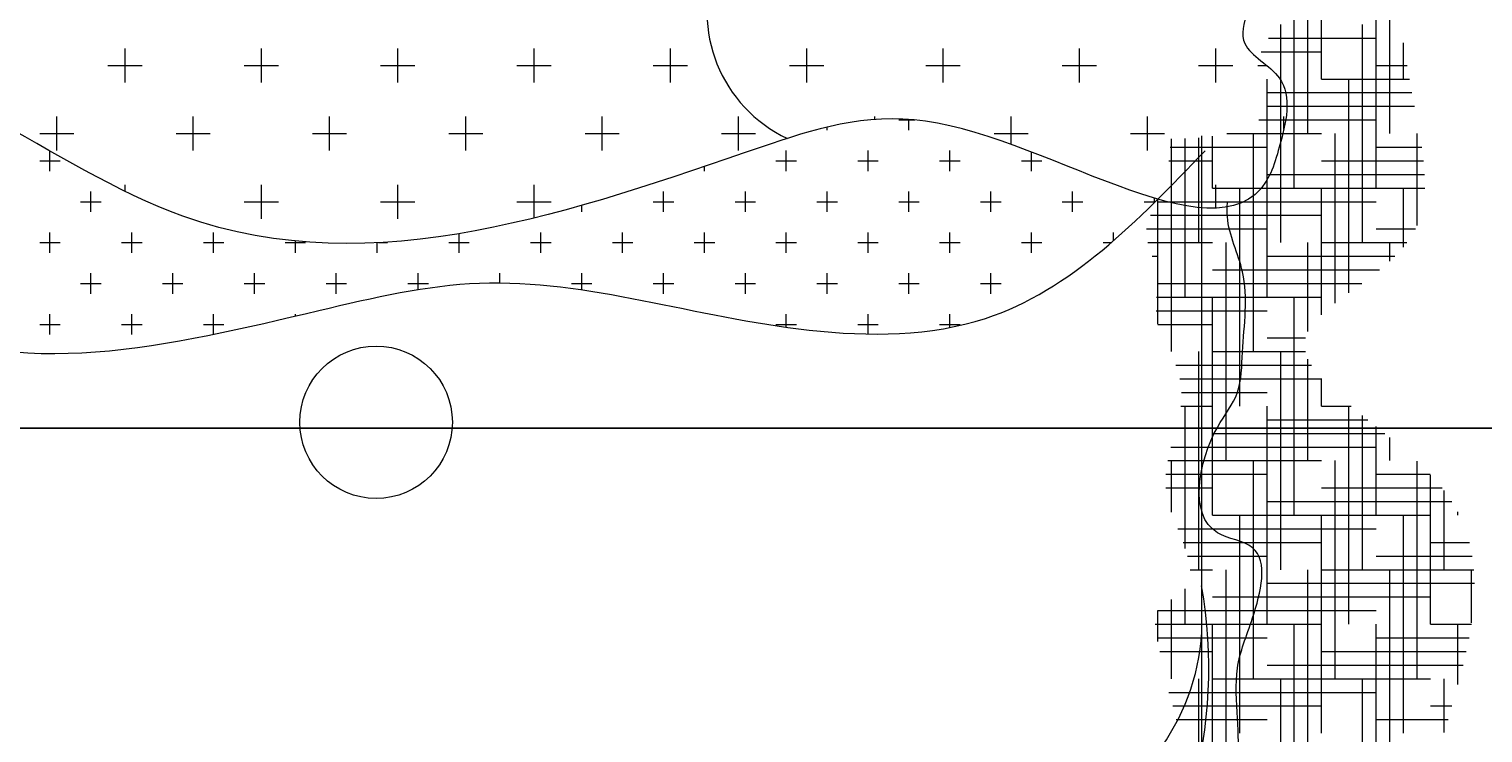
# Model space of a CAD drawing. Units: inches. Extents: x 2330 to 3943, y 1763 to 3461.
# Tile 34 of 40: x 3347 to 3417, y 3064 to 3098. Entities that reach past the tile are written whole.
import ezdxf

# ---------------------------------------------------------------- set-up
doc = ezdxf.new("R2010")
doc.units = ezdxf.units.IN
doc.layers.add('A-ANNO-DIMS', color=2, linetype='Continuous', lineweight=18)
doc.layers.add('A-FURN', color=8, linetype='Continuous', lineweight=13)
doc.styles.get("Standard").update_dxf_attribs({"font": 'arial.ttf'})
doc.dimstyles.get("Standard").update_dxf_attribs({"dimtxt": 0.18, "dimasz": 0.18, "dimexe": 0.18, "dimexo": 0.0625, "dimgap": 0.09, "dimtad": 0, "dimtih": 1, "dimtoh": 1, "dimdec": 4, "dimzin": 0, "dimdsep": 46, "dimtxsty": 'Standard', "dimcen": 0.09, "dimadec": 0, "dimazin": 0, "dimtfac": 1, "dimtdec": 4, "dimtofl": 0, "dimtmove": 0, "dimatfit": 3, "dimfxl": 1, "dimtolj": 1, "dimtzin": 0, "dimarcsym": 0})

# ---------------------------------------------------------------- blocks, each defined once
blk = doc.blocks.new('A$C200C7901')
at = {"linetype": 'ByBlock'}
for p, q in [((2.0974, 1.2977), (2.0974, 1.4977)), ((2.0974, 1.2977), (2.0974, 1.4977)), ((2.1099, 1.3477), (2.1099, 1.5009)), ((2.1099, 1.3477), (2.1099, 1.5009)), ((2.1599, 1.2477), (2.1599, 1.4477)), ((2.1599, 1.2477), (2.1599, 1.4477)), ((2.1724, 1.2977), (2.1724, 1.439)), ((2.1724, 1.2977), (2.1724, 1.439)), ((2.0849, 1.2477), (2.0849, 1.4171)), ((2.0849, 1.2477), (2.0849, 1.4171)), ((2.0724, 1.1977), (2.0724, 1.3977)), ((2.0724, 1.1977), (2.0724, 1.3977)), ((2.1474, 1.1977), (2.1474, 1.3977)), ((2.1474, 1.1977), (2.1474, 1.3977)), ((1.0129, 1.3445), (1.0129, 1.3758)), ((1.0129, 1.3445), (1.0129, 1.3758)), ((1.1379, 1.3445), (1.1379, 1.3758)), ((1.1379, 1.3445), (1.1379, 1.3758)), ((1.2629, 1.3445), (1.2629, 1.3758)), ((1.2629, 1.3445), (1.2629, 1.3758)), ((1.3879, 1.3445), (1.3879, 1.3758)), ((1.3879, 1.3445), (1.3879, 1.3758)), ((1.5129, 1.3445), (1.5129, 1.3758)), ((1.5129, 1.3445), (1.5129, 1.3758)), ((1.6379, 1.3445), (1.6379, 1.3758)), ((1.6379, 1.3445), (1.6379, 1.3758)), ((1.7629, 1.3445), (1.7629, 1.3758)), ((1.7629, 1.3445), (1.7629, 1.3758)), ((1.8879, 1.3445), (1.8879, 1.3758)), ((1.8879, 1.3445), (1.8879, 1.3758)), ((2.0129, 1.3445), (2.0129, 1.3758)), ((2.0129, 1.3445), (2.0129, 1.3758)), ((2.0612, 1.3852), (2.1599, 1.3852)), ((2.0612, 1.3852), (2.1599, 1.3852)), ((2.1849, 1.3477), (2.1849, 1.3808)), ((2.1849, 1.3477), (2.1849, 1.3808)), ((0.9972, 1.3602), (1.0285, 1.3602)), ((0.9972, 1.3602), (1.0285, 1.3602)), ((1.1222, 1.3602), (1.1535, 1.3602)), ((1.1222, 1.3602), (1.1535, 1.3602)), ((1.2472, 1.3602), (1.2785, 1.3602)), ((1.2472, 1.3602), (1.2785, 1.3602)), ((1.3722, 1.3602), (1.4035, 1.3602)), ((1.3722, 1.3602), (1.4035, 1.3602)), ((1.4972, 1.3602), (1.5285, 1.3602)), ((1.4972, 1.3602), (1.5285, 1.3602)), ((1.6222, 1.3602), (1.6535, 1.3602)), ((1.6222, 1.3602), (1.6535, 1.3602)), ((1.7472, 1.3602), (1.7785, 1.3602)), ((1.7472, 1.3602), (1.7785, 1.3602)), ((1.8722, 1.3602), (1.9035, 1.3602)), ((1.8722, 1.3602), (1.9035, 1.3602)), ((1.9972, 1.3602), (2.0285, 1.3602)), ((1.9972, 1.3602), (2.0285, 1.3602)), ((2.0515, 1.3602), (2.0599, 1.3602)), ((2.0515, 1.3602), (2.0599, 1.3602)), ((2.0545, 1.3727), (2.1099, 1.3727)), ((2.0545, 1.3727), (2.1099, 1.3727)), ((2.1599, 1.3602), (2.1883, 1.3602)), ((2.1599, 1.3602), (2.1883, 1.3602)), ((2.0599, 1.1477), (2.0599, 1.3477)), ((2.0599, 1.1477), (2.0599, 1.3477)), ((2.1099, 1.3477), (2.1904, 1.3477)), ((2.1099, 1.3477), (2.1904, 1.3477)), ((2.1349, 1.1515), (2.1349, 1.3477)), ((2.1349, 1.1515), (2.1349, 1.3477)), ((2.0599, 1.3352), (2.1926, 1.3352)), ((2.0599, 1.3352), (2.1926, 1.3352)), ((2.0594, 1.3227), (2.195, 1.3227)), ((2.0594, 1.3227), (2.195, 1.3227)), ((0.9504, 1.282), (0.9504, 1.3133)), ((0.9504, 1.282), (0.9504, 1.3133)), ((1.0754, 1.282), (1.0754, 1.3133)), ((1.0754, 1.282), (1.0754, 1.3133)), ((1.2004, 1.282), (1.2004, 1.3133)), ((1.2004, 1.282), (1.2004, 1.3133)), ((1.3254, 1.282), (1.3254, 1.3133)), ((1.3254, 1.282), (1.3254, 1.3133)), ((1.4504, 1.282), (1.4504, 1.3133)), ((1.4504, 1.282), (1.4504, 1.3133)), ((1.5754, 1.282), (1.5754, 1.3133)), ((1.5754, 1.282), (1.5754, 1.3133)), ((1.7004, 1.3106), (1.7004, 1.3133)), ((1.7004, 1.3106), (1.7004, 1.3133)), ((1.7222, 1.3102), (1.7369, 1.3102)), ((1.7222, 1.3102), (1.7369, 1.3102)), ((1.7316, 1.3008), (1.7316, 1.3106)), ((1.7316, 1.3008), (1.7316, 1.3106)), ((1.8254, 1.2876), (1.8254, 1.3133)), ((1.8254, 1.2876), (1.8254, 1.3133)), ((1.9504, 1.282), (1.9504, 1.3133)), ((1.9504, 1.282), (1.9504, 1.3133)), ((2.0524, 1.3102), (2.1599, 1.3102)), ((2.0524, 1.3102), (2.1599, 1.3102)), ((2.0754, 1.3017), (2.0754, 1.3133)), ((2.0754, 1.3017), (2.0754, 1.3133)), ((0.9347, 1.2977), (0.966, 1.2977)), ((0.9347, 1.2977), (0.966, 1.2977)), ((1.0597, 1.2977), (1.091, 1.2977)), ((1.0597, 1.2977), (1.091, 1.2977)), ((1.1847, 1.2977), (1.216, 1.2977)), ((1.1847, 1.2977), (1.216, 1.2977)), ((1.3097, 1.2977), (1.341, 1.2977)), ((1.3097, 1.2977), (1.341, 1.2977)), ((1.4347, 1.2977), (1.466, 1.2977)), ((1.4347, 1.2977), (1.466, 1.2977)), ((1.5597, 1.2977), (1.591, 1.2977)), ((1.5597, 1.2977), (1.591, 1.2977)), ((1.6566, 1.3008), (1.6566, 1.3036)), ((1.6566, 1.3008), (1.6566, 1.3036)), ((1.8097, 1.2977), (1.841, 1.2977)), ((1.8097, 1.2977), (1.841, 1.2977)), ((1.9347, 1.2977), (1.966, 1.2977)), ((1.9347, 1.2977), (1.966, 1.2977)), ((1.9849, 1.1477), (1.9849, 1.293)), ((1.9849, 1.1477), (1.9849, 1.293)), ((1.9974, 1.1977), (1.9974, 1.2939)), ((1.9974, 1.1977), (1.9974, 1.2939)), ((2.0099, 1.2477), (2.0099, 1.2953)), ((2.0099, 1.2477), (2.0099, 1.2953)), ((2.023, 1.2977), (2.1099, 1.2977)), ((2.023, 1.2977), (2.1099, 1.2977)), ((2.0474, 1.0977), (2.0474, 1.2977)), ((2.0474, 1.0977), (2.0474, 1.2977)), ((2.0597, 1.2977), (2.0744, 1.2977)), ((2.0597, 1.2977), (2.0744, 1.2977)), ((2.1224, 1.1421), (2.1224, 1.2977)), ((2.1224, 1.1421), (2.1224, 1.2977)), ((2.1974, 1.2135), (2.1974, 1.2977)), ((2.1974, 1.2135), (2.1974, 1.2977)), ((0.9441, 1.2633), (0.9441, 1.2816)), ((0.9441, 1.2633), (0.9441, 1.2816)), ((1.6191, 1.2633), (1.6191, 1.282)), ((1.6191, 1.2633), (1.6191, 1.282)), ((1.6941, 1.2633), (1.6941, 1.282)), ((1.6941, 1.2633), (1.6941, 1.282)), ((1.7691, 1.2633), (1.7691, 1.282)), ((1.7691, 1.2633), (1.7691, 1.282)), ((1.8441, 1.2633), (1.8441, 1.2806)), ((1.8441, 1.2633), (1.8441, 1.2806)), ((1.9711, 1.2852), (2.0599, 1.2852)), ((1.9711, 1.2852), (2.0599, 1.2852)), ((1.9724, 1.0977), (1.9724, 1.2927)), ((1.9724, 1.0977), (1.9724, 1.2927)), ((2.1599, 1.2852), (2.2018, 1.2852)), ((2.1599, 1.2852), (2.2018, 1.2852)), ((0.9347, 1.2727), (0.9535, 1.2727)), ((0.9347, 1.2727), (0.9535, 1.2727)), ((1.5441, 1.2633), (1.5441, 1.2675)), ((1.5441, 1.2633), (1.5441, 1.2675)), ((1.6097, 1.2727), (1.6285, 1.2727)), ((1.6097, 1.2727), (1.6285, 1.2727)), ((1.6847, 1.2727), (1.7035, 1.2727)), ((1.6847, 1.2727), (1.7035, 1.2727)), ((1.7597, 1.2727), (1.7785, 1.2727)), ((1.7597, 1.2727), (1.7785, 1.2727)), ((1.8347, 1.2727), (1.8535, 1.2727)), ((1.8347, 1.2727), (1.8535, 1.2727)), ((1.97, 1.2727), (2.0099, 1.2727)), ((1.97, 1.2727), (2.0099, 1.2727)), ((2.1099, 1.2727), (2.2034, 1.2727)), ((2.1099, 1.2727), (2.2034, 1.2727)), ((2.0599, 1.2602), (2.2044, 1.2602)), ((2.0599, 1.2602), (2.2044, 1.2602)), ((0.9816, 1.2258), (0.9816, 1.2445)), ((0.9816, 1.2258), (0.9816, 1.2445)), ((1.0129, 1.2448), (1.0129, 1.2508)), ((1.0129, 1.2448), (1.0129, 1.2508)), ((1.1379, 1.2195), (1.1379, 1.2508)), ((1.1379, 1.2195), (1.1379, 1.2508)), ((1.2629, 1.2195), (1.2629, 1.2508)), ((1.2629, 1.2195), (1.2629, 1.2508)), ((1.3879, 1.2202), (1.3879, 1.2508)), ((1.3879, 1.2202), (1.3879, 1.2508)), ((1.5066, 1.2258), (1.5066, 1.2445)), ((1.5066, 1.2258), (1.5066, 1.2445)), ((1.5816, 1.2258), (1.5816, 1.2445)), ((1.5816, 1.2258), (1.5816, 1.2445)), ((1.6566, 1.2258), (1.6566, 1.2445)), ((1.6566, 1.2258), (1.6566, 1.2445)), ((1.7316, 1.2258), (1.7316, 1.2445)), ((1.7316, 1.2258), (1.7316, 1.2445)), ((1.8066, 1.2258), (1.8066, 1.2445)), ((1.8066, 1.2258), (1.8066, 1.2445)), ((1.8816, 1.2258), (1.8816, 1.2445)), ((1.8816, 1.2258), (1.8816, 1.2445)), ((2.0099, 1.2477), (2.2045, 1.2477)), ((2.0099, 1.2477), (2.2045, 1.2477)), ((2.0129, 1.2293), (2.0129, 1.2508)), ((2.0129, 1.2293), (2.0129, 1.2508)), ((2.0349, 1.0477), (2.0349, 1.2477)), ((2.0349, 1.0477), (2.0349, 1.2477)), ((2.1099, 1.1315), (2.1099, 1.2477)), ((2.1099, 1.1315), (2.1099, 1.2477)), ((2.1849, 1.1935), (2.1849, 1.2477)), ((2.1849, 1.1935), (2.1849, 1.2477)), ((0.9722, 1.2352), (0.991, 1.2352)), ((0.9722, 1.2352), (0.991, 1.2352)), ((1.1222, 1.2352), (1.1535, 1.2352)), ((1.1222, 1.2352), (1.1535, 1.2352)), ((1.2472, 1.2352), (1.2785, 1.2352)), ((1.2472, 1.2352), (1.2785, 1.2352)), ((1.3722, 1.2352), (1.4035, 1.2352)), ((1.3722, 1.2352), (1.4035, 1.2352)), ((1.4316, 1.2258), (1.4316, 1.2318)), ((1.4316, 1.2258), (1.4316, 1.2318)), ((1.4972, 1.2352), (1.516, 1.2352)), ((1.4972, 1.2352), (1.516, 1.2352)), ((1.5722, 1.2352), (1.591, 1.2352)), ((1.5722, 1.2352), (1.591, 1.2352)), ((1.6472, 1.2352), (1.666, 1.2352)), ((1.6472, 1.2352), (1.666, 1.2352)), ((1.7222, 1.2352), (1.741, 1.2352)), ((1.7222, 1.2352), (1.741, 1.2352)), ((1.7972, 1.2352), (1.816, 1.2352)), ((1.7972, 1.2352), (1.816, 1.2352)), ((1.8722, 1.2352), (1.891, 1.2352)), ((1.8722, 1.2352), (1.891, 1.2352)), ((1.9472, 1.2352), (1.9574, 1.2352)), ((1.9472, 1.2352), (1.9574, 1.2352)), ((1.9566, 1.2344), (1.9566, 1.2385)), ((1.9566, 1.2344), (1.9566, 1.2385)), ((1.9599, 1.1228), (1.9599, 1.2373)), ((1.9599, 1.1228), (1.9599, 1.2373)), ((1.9599, 1.2352), (2.1599, 1.2352)), ((1.9599, 1.2352), (2.1599, 1.2352)), ((2, 1.2352), (2.0285, 1.2352)), ((2, 1.2352), (2.0285, 1.2352)), ((1.953, 1.2227), (2.1099, 1.2227)), ((1.953, 1.2227), (2.1099, 1.2227)), ((0.9441, 1.1883), (0.9441, 1.207)), ((0.9441, 1.1883), (0.9441, 1.207)), ((1.0191, 1.1883), (1.0191, 1.207)), ((1.0191, 1.1883), (1.0191, 1.207)), ((1.0941, 1.1883), (1.0941, 1.207)), ((1.0941, 1.1883), (1.0941, 1.207)), ((1.3191, 1.1883), (1.3191, 1.2059)), ((1.3191, 1.1883), (1.3191, 1.2059)), ((1.3941, 1.1883), (1.3941, 1.207)), ((1.3941, 1.1883), (1.3941, 1.207)), ((1.4691, 1.1883), (1.4691, 1.207)), ((1.4691, 1.1883), (1.4691, 1.207)), ((1.5441, 1.1883), (1.5441, 1.207)), ((1.5441, 1.1883), (1.5441, 1.207)), ((1.6191, 1.1883), (1.6191, 1.207)), ((1.6191, 1.1883), (1.6191, 1.207)), ((1.6941, 1.1883), (1.6941, 1.207)), ((1.6941, 1.1883), (1.6941, 1.207)), ((1.7691, 1.1883), (1.7691, 1.207)), ((1.7691, 1.1883), (1.7691, 1.207)), ((1.8441, 1.1883), (1.8441, 1.207)), ((1.8441, 1.1883), (1.8441, 1.207)), ((1.9191, 1.1995), (1.9191, 1.207)), ((1.9191, 1.1995), (1.9191, 1.207)), ((1.9495, 1.2102), (2.0599, 1.2102)), ((1.9495, 1.2102), (2.0599, 1.2102)), ((2.1599, 1.2102), (2.1959, 1.2102)), ((2.1599, 1.2102), (2.1959, 1.2102)), ((0.9347, 1.1977), (0.9535, 1.1977)), ((0.9347, 1.1977), (0.9535, 1.1977)), ((1.0097, 1.1977), (1.0285, 1.1977)), ((1.0097, 1.1977), (1.0285, 1.1977)), ((1.0847, 1.1977), (1.1035, 1.1977)), ((1.0847, 1.1977), (1.1035, 1.1977)), ((1.1597, 1.1977), (1.1785, 1.1977)), ((1.1597, 1.1977), (1.1785, 1.1977)), ((1.1691, 1.1883), (1.1691, 1.1991)), ((1.1691, 1.1883), (1.1691, 1.1991)), ((1.2441, 1.1883), (1.2441, 1.1976)), ((1.2441, 1.1883), (1.2441, 1.1976)), ((1.2452, 1.1977), (1.2535, 1.1977)), ((1.2452, 1.1977), (1.2535, 1.1977)), ((1.3097, 1.1977), (1.3285, 1.1977)), ((1.3097, 1.1977), (1.3285, 1.1977)), ((1.3847, 1.1977), (1.4035, 1.1977)), ((1.3847, 1.1977), (1.4035, 1.1977)), ((1.4597, 1.1977), (1.4785, 1.1977)), ((1.4597, 1.1977), (1.4785, 1.1977)), ((1.5347, 1.1977), (1.5535, 1.1977)), ((1.5347, 1.1977), (1.5535, 1.1977)), ((1.6097, 1.1977), (1.6285, 1.1977)), ((1.6097, 1.1977), (1.6285, 1.1977)), ((1.6847, 1.1977), (1.7035, 1.1977)), ((1.6847, 1.1977), (1.7035, 1.1977)), ((1.7597, 1.1977), (1.7785, 1.1977)), ((1.7597, 1.1977), (1.7785, 1.1977)), ((1.8347, 1.1977), (1.8535, 1.1977)), ((1.8347, 1.1977), (1.8535, 1.1977)), ((1.9097, 1.1977), (1.917, 1.1977)), ((1.9097, 1.1977), (1.917, 1.1977)), ((1.9506, 1.1977), (2.0099, 1.1977)), ((1.9506, 1.1977), (2.0099, 1.1977)), ((2.0974, 1.1161), (2.0974, 1.1977)), ((2.0974, 1.1161), (2.0974, 1.1977)), ((2.1099, 1.1977), (2.1882, 1.1977)), ((2.1099, 1.1977), (2.1882, 1.1977)), ((2.1724, 1.1807), (2.1724, 1.1977)), ((2.1724, 1.1807), (2.1724, 1.1977)), ((1.9545, 1.1852), (1.9599, 1.1852)), ((1.9545, 1.1852), (1.9599, 1.1852)), ((2.0599, 1.1852), (2.1772, 1.1852)), ((2.0599, 1.1852), (2.1772, 1.1852)), ((0.9722, 1.1602), (0.991, 1.1602)), ((0.9722, 1.1602), (0.991, 1.1602)), ((0.9816, 1.1508), (0.9816, 1.1695)), ((0.9816, 1.1508), (0.9816, 1.1695)), ((1.0472, 1.1602), (1.066, 1.1602)), ((1.0472, 1.1602), (1.066, 1.1602)), ((1.0566, 1.1508), (1.0566, 1.1695)), ((1.0566, 1.1508), (1.0566, 1.1695)), ((1.1222, 1.1602), (1.141, 1.1602)), ((1.1222, 1.1602), (1.141, 1.1602)), ((1.1316, 1.1508), (1.1316, 1.1695)), ((1.1316, 1.1508), (1.1316, 1.1695)), ((1.1972, 1.1602), (1.216, 1.1602)), ((1.1972, 1.1602), (1.216, 1.1602)), ((1.2066, 1.1508), (1.2066, 1.1695)), ((1.2066, 1.1508), (1.2066, 1.1695)), ((1.2722, 1.1602), (1.291, 1.1602)), ((1.2722, 1.1602), (1.291, 1.1602)), ((1.2816, 1.1547), (1.2816, 1.1695)), ((1.2816, 1.1547), (1.2816, 1.1695)), ((1.3566, 1.1608), (1.3566, 1.1695)), ((1.3566, 1.1608), (1.3566, 1.1695)), ((1.4222, 1.1602), (1.441, 1.1602)), ((1.4222, 1.1602), (1.441, 1.1602)), ((1.4316, 1.1544), (1.4316, 1.1695)), ((1.4316, 1.1544), (1.4316, 1.1695)), ((1.4972, 1.1602), (1.516, 1.1602)), ((1.4972, 1.1602), (1.516, 1.1602)), ((1.5066, 1.1508), (1.5066, 1.1695)), ((1.5066, 1.1508), (1.5066, 1.1695)), ((1.5722, 1.1602), (1.591, 1.1602)), ((1.5722, 1.1602), (1.591, 1.1602)), ((1.5816, 1.1508), (1.5816, 1.1695)), ((1.5816, 1.1508), (1.5816, 1.1695)), ((1.6472, 1.1602), (1.666, 1.1602)), ((1.6472, 1.1602), (1.666, 1.1602)), ((1.6566, 1.1508), (1.6566, 1.1695)), ((1.6566, 1.1508), (1.6566, 1.1695)), ((1.7222, 1.1602), (1.741, 1.1602)), ((1.7222, 1.1602), (1.741, 1.1602)), ((1.7316, 1.1508), (1.7316, 1.1695)), ((1.7316, 1.1508), (1.7316, 1.1695)), ((1.7972, 1.1602), (1.816, 1.1602)), ((1.7972, 1.1602), (1.816, 1.1602)), ((1.8066, 1.1508), (1.8066, 1.1695)), ((1.8066, 1.1508), (1.8066, 1.1695)), ((1.9599, 1.1602), (2.1468, 1.1602)), ((1.9599, 1.1602), (2.1468, 1.1602)), ((2.0099, 1.1727), (2.1631, 1.1727)), ((2.0099, 1.1727), (2.1631, 1.1727)), ((1.9585, 1.1477), (2.1099, 1.1477)), ((1.9585, 1.1477), (2.1099, 1.1477)), ((2.0099, 0.9477), (2.0099, 1.1477)), ((2.0099, 0.9477), (2.0099, 1.1477)), ((2.0849, 0.9477), (2.0849, 1.1477)), ((2.0849, 0.9477), (2.0849, 1.1477)), ((1.9581, 1.1352), (2.0599, 1.1352)), ((1.9581, 1.1352), (2.0599, 1.1352)), ((0.9347, 1.1227), (0.9535, 1.1227)), ((0.9347, 1.1227), (0.9535, 1.1227)), ((0.9441, 1.1133), (0.9441, 1.132)), ((0.9441, 1.1133), (0.9441, 1.132)), ((1.0097, 1.1227), (1.0285, 1.1227)), ((1.0097, 1.1227), (1.0285, 1.1227)), ((1.0191, 1.1133), (1.0191, 1.132)), ((1.0191, 1.1133), (1.0191, 1.132)), ((1.0847, 1.1227), (1.1035, 1.1227)), ((1.0847, 1.1227), (1.1035, 1.1227)), ((1.0941, 1.1136), (1.0941, 1.132)), ((1.0941, 1.1136), (1.0941, 1.132)), ((1.1691, 1.1303), (1.1691, 1.132)), ((1.1691, 1.1303), (1.1691, 1.132)), ((1.6097, 1.1227), (1.6285, 1.1227)), ((1.6097, 1.1227), (1.6285, 1.1227)), ((1.6191, 1.1201), (1.6191, 1.132)), ((1.6191, 1.1201), (1.6191, 1.132)), ((1.6847, 1.1227), (1.7035, 1.1227)), ((1.6847, 1.1227), (1.7035, 1.1227)), ((1.6941, 1.1139), (1.6941, 1.132)), ((1.6941, 1.1139), (1.6941, 1.132)), ((1.7597, 1.1227), (1.7785, 1.1227)), ((1.7597, 1.1227), (1.7785, 1.1227)), ((1.7691, 1.1198), (1.7691, 1.132)), ((1.7691, 1.1198), (1.7691, 1.132)), ((1.9599, 1.1227), (2.0099, 1.1227)), ((1.9599, 1.1227), (2.0099, 1.1227)), ((2.0599, 1.1102), (2.0951, 1.1102)), ((2.0599, 1.1102), (2.0951, 1.1102)), ((1.9974, 0.8977), (1.9974, 1.0977)), ((1.9974, 0.8977), (1.9974, 1.0977)), ((2.0099, 1.0977), (2.095, 1.0977)), ((2.0099, 1.0977), (2.095, 1.0977)), ((2.0724, 0.8977), (2.0724, 1.0977)), ((2.0724, 0.8977), (2.0724, 1.0977)), ((1.9763, 1.0852), (2.1005, 1.0852)), ((1.9763, 1.0852), (2.1005, 1.0852)), ((2.0974, 0.9977), (2.0974, 1.0909)), ((2.0974, 0.9977), (2.0974, 1.0909)), ((1.9799, 1.0727), (2.1099, 1.0727)), ((1.9799, 1.0727), (2.1099, 1.0727)), ((2.1099, 1.0477), (2.1099, 1.0729)), ((2.1099, 1.0477), (2.1099, 1.0729)), ((1.9815, 1.0602), (2.0599, 1.0602)), ((1.9815, 1.0602), (2.0599, 1.0602)), ((1.981, 1.0477), (2.0099, 1.0477)), ((1.981, 1.0477), (2.0099, 1.0477)), ((1.9849, 0.9171), (1.9849, 1.0477)), ((1.9849, 0.9171), (1.9849, 1.0477)), ((2.0599, 0.8477), (2.0599, 1.0477)), ((2.0599, 0.8477), (2.0599, 1.0477)), ((2.1099, 1.0477), (2.137, 1.0477)), ((2.1099, 1.0477), (2.137, 1.0477)), ((2.1349, 0.8477), (2.1349, 1.0477)), ((2.1349, 0.8477), (2.1349, 1.0477)), ((2.0599, 1.0352), (2.1523, 1.0352)), ((2.0599, 1.0352), (2.1523, 1.0352)), ((2.1474, 0.8977), (2.1474, 1.0391)), ((2.1474, 0.8977), (2.1474, 1.0391)), ((2.1599, 0.9477), (2.1599, 1.029)), ((2.1599, 0.9477), (2.1599, 1.029)), ((2.0099, 1.0227), (2.1678, 1.0227)), ((2.0099, 1.0227), (2.1678, 1.0227)), ((2.1724, 0.9977), (2.1724, 1.0189)), ((2.1724, 0.9977), (2.1724, 1.0189)), ((1.9718, 1.0102), (2.1599, 1.0102)), ((1.9718, 1.0102), (2.1599, 1.0102)), ((1.9688, 0.9977), (2.1099, 0.9977)), ((1.9688, 0.9977), (2.1099, 0.9977)), ((1.9724, 0.9504), (1.9724, 0.9977)), ((1.9724, 0.9504), (1.9724, 0.9977)), ((2.0474, 0.7977), (2.0474, 0.9977)), ((2.0474, 0.7977), (2.0474, 0.9977)), ((2.1224, 0.7977), (2.1224, 0.9977)), ((2.1224, 0.7977), (2.1224, 0.9977)), ((2.1974, 0.7977), (2.1974, 0.9972)), ((2.1974, 0.7977), (2.1974, 0.9972)), ((1.9671, 0.9852), (2.0599, 0.9852)), ((1.9671, 0.9852), (2.0599, 0.9852)), ((2.1599, 0.9852), (2.2095, 0.9852)), ((2.1599, 0.9852), (2.2095, 0.9852)), ((2.2099, 0.8477), (2.2099, 0.9848)), ((2.2099, 0.8477), (2.2099, 0.9848)), ((1.9672, 0.9727), (2.0099, 0.9727)), ((1.9672, 0.9727), (2.0099, 0.9727)), ((2.0599, 0.9602), (2.2294, 0.9602)), ((2.0599, 0.9602), (2.2294, 0.9602)), ((2.1099, 0.9727), (2.2204, 0.9727)), ((2.1099, 0.9727), (2.2204, 0.9727)), ((2.2224, 0.8977), (2.2224, 0.9702)), ((2.2224, 0.8977), (2.2224, 0.9702)), ((2.0099, 0.9477), (2.2099, 0.9477)), ((2.0099, 0.9477), (2.2099, 0.9477)), ((2.0349, 0.7477), (2.0349, 0.9477)), ((2.0349, 0.7477), (2.0349, 0.9477)), ((2.1099, 0.7477), (2.1099, 0.9477)), ((2.1099, 0.7477), (2.1099, 0.9477)), ((2.1849, 0.7477), (2.1849, 0.9477)), ((2.1849, 0.7477), (2.1849, 0.9477)), ((2.2349, 0.9477), (2.2349, 0.9506)), ((2.2349, 0.9477), (2.2349, 0.9506)), ((1.9781, 0.9352), (2.1599, 0.9352)), ((1.9781, 0.9352), (2.1599, 0.9352)), ((1.9829, 0.9227), (2.1099, 0.9227)), ((1.9829, 0.9227), (2.1099, 0.9227)), ((2.2099, 0.9227), (2.2455, 0.9227)), ((2.2099, 0.9227), (2.2455, 0.9227)), ((1.9871, 0.9102), (2.0599, 0.9102)), ((1.9871, 0.9102), (2.0599, 0.9102)), ((2.1599, 0.9102), (2.2481, 0.9102)), ((2.1599, 0.9102), (2.2481, 0.9102)), ((1.9894, 0.8977), (2.0099, 0.8977)), ((1.9894, 0.8977), (2.0099, 0.8977)), ((2.0224, 0.6977), (2.0224, 0.8977)), ((2.0224, 0.6977), (2.0224, 0.8977)), ((2.0974, 0.6977), (2.0974, 0.8977)), ((2.0974, 0.6977), (2.0974, 0.8977)), ((2.1099, 0.8977), (2.2496, 0.8977)), ((2.1099, 0.8977), (2.2496, 0.8977)), ((2.1724, 0.6977), (2.1724, 0.8977)), ((2.1724, 0.6977), (2.1724, 0.8977)), ((2.2474, 0.8489), (2.2474, 0.8977)), ((2.2474, 0.8489), (2.2474, 0.8977)), ((1.9849, 0.8477), (1.9849, 0.88)), ((1.9849, 0.8477), (1.9849, 0.88)), ((2.0599, 0.8852), (2.2501, 0.8852)), ((2.0599, 0.8852), (2.2501, 0.8852)), ((1.9724, 0.7977), (1.9724, 0.8703)), ((1.9724, 0.7977), (1.9724, 0.8703)), ((2.0099, 0.8727), (2.2099, 0.8727)), ((2.0099, 0.8727), (2.2099, 0.8727)), ((1.9599, 0.8317), (1.9599, 0.8604)), ((1.9599, 0.8317), (1.9599, 0.8604)), ((1.9599, 0.8602), (2.1599, 0.8602)), ((1.9599, 0.8602), (2.1599, 0.8602)), ((1.9574, 0.8477), (2.1099, 0.8477)), ((1.9574, 0.8477), (2.1099, 0.8477)), ((2.0099, 0.6477), (2.0099, 0.8477)), ((2.0099, 0.6477), (2.0099, 0.8477)), ((2.0849, 0.6477), (2.0849, 0.8477)), ((2.0849, 0.6477), (2.0849, 0.8477)), ((2.1599, 0.6477), (2.1599, 0.8477)), ((2.1599, 0.6477), (2.1599, 0.8477)), ((2.2099, 0.8477), (2.2472, 0.8477)), ((2.2099, 0.8477), (2.2472, 0.8477)), ((2.2349, 0.7923), (2.2349, 0.8477)), ((2.2349, 0.7923), (2.2349, 0.8477)), ((1.9593, 0.8352), (2.0599, 0.8352)), ((1.9593, 0.8352), (2.0599, 0.8352)), ((2.1599, 0.8352), (2.2451, 0.8352)), ((2.1599, 0.8352), (2.2451, 0.8352)), ((1.9615, 0.8227), (2.0099, 0.8227)), ((1.9615, 0.8227), (2.0099, 0.8227)), ((2.1099, 0.8227), (2.2425, 0.8227)), ((2.1099, 0.8227), (2.2425, 0.8227)), ((2.0599, 0.8102), (2.2396, 0.8102)), ((2.0599, 0.8102), (2.2396, 0.8102)), ((2.0099, 0.7977), (2.2099, 0.7977)), ((2.0099, 0.7977), (2.2099, 0.7977)), ((2.2224, 0.7483), (2.2224, 0.7977)), ((2.2224, 0.7483), (2.2224, 0.7977)), ((1.9699, 0.7852), (2.1599, 0.7852)), ((1.9699, 0.7852), (2.1599, 0.7852)), ((1.9734, 0.7727), (2.1099, 0.7727)), ((1.9734, 0.7727), (2.1099, 0.7727)), ((1.9767, 0.7602), (2.0599, 0.7602)), ((1.9767, 0.7602), (2.0599, 0.7602)), ((2.1599, 0.7602), (2.2258, 0.7602)), ((2.1599, 0.7602), (2.2258, 0.7602)), ((2.2099, 0.7727), (2.2294, 0.7727)), ((2.2099, 0.7727), (2.2294, 0.7727))]:
    blk.add_line(p, q, dxfattribs=at)
for p, q in [((2, 0.2957), (2, 1.2957)), ((2.0224, 0.9977), (2.0224, 1.1977)), ((2.0224, 0.9977), (2.0224, 1.1977)), ((1.9974, 0.5977), (1.9974, 0.7977)), ((1.9974, 0.5977), (1.9974, 0.7977)), ((2.0724, 0.5977), (2.0724, 0.7977)), ((2.0724, 0.5977), (2.0724, 0.7977)), ((2.1474, 0.5977), (2.1474, 0.7977)), ((2.1474, 0.5977), (2.1474, 0.7977))]:
    blk.add_line(p, q)
blk.add_circle((1.2431, 1.0329), 0.0699)
blk.add_arc((1.6746, 1.4093), 0.1282, 72.7909, 244.8695, dxfattribs=at)
blk.add_arc((1.6746, 1.4093), 0.1282, 72.7909, 244.8695, dxfattribs=at)
for centre, radius, start, end in [((1.5693, 0.8075), 0.4372, 269.0679, 9.9322), ((1.7969, 0.8525), 0.2035, 222.1514, 356.4639)]:
    blk.add_arc(centre, radius, start, end)
for points, knots in [([(0.4485, 1.7835), (0.4321, 1.7496), (0.4062, 1.6964), (0.49, 1.6713), (0.4719, 1.5969), (0.4123, 1.592), (0.4233, 1.5337), (0.4954, 1.5086), (0.4012, 1.4738), (0.3253, 1.4306), (0.4113, 1.3764), (0.3688, 1.3065), (0.5579, 1.2663), (0.741, 1.4533), (1.1127, 1.1109), (1.4811, 1.2478), (1.7885, 1.3492), (2.0357, 1.1637), (2.0748, 1.2974), (2.0876, 1.349), (2.0192, 1.3805), (2.0564, 1.4298), (2.0588, 1.4846), (1.9759, 1.5349), (2.1004, 1.5845), (2.0397, 1.6519), (1.971, 1.7053), (2.1104, 1.8981), (1.5946, 1.7967), (1.2448, 1.7472), (0.8129, 1.7935), (0.4953, 1.8548), (0.4582, 1.7983), (0.4485, 1.7835)], [0, 0, 0, 0, 88.420092, 139.08588, 204.302936, 239.695496, 287.801042, 327.365471, 412.960499, 463.626286, 552.059846, 584.668336, 662.614915, 940.993281, 1309.926334, 1844.022653, 1996.276242, 2316.43048, 2341.441004, 2404.707416, 2449.463774, 2514.680778, 2538.40571, 2613.031547, 2697.13096, 2760.903931, 2822.692699, 2945.47, 3215.060018, 3725.584917, 4361.974444, 4504.671998, 4555.32777, 4555.32777, 4555.32777, 4555.32777]), ([(0.4856, 1.3429), (0.5504, 1.3182), (0.6715, 1.2721), (0.8374, 1.0498), (1.1164, 1.1183), (1.3878, 1.1816), (1.5888, 1.1102), (1.8403, 1.1127), (1.9415, 1.2178), (2.0032, 1.2819)], [0, 0, 0, 0, 205.411753, 383.654933, 772.067458, 921.644661, 1226.793228, 1388.983508, 1642.292305, 1642.292305, 1642.292305, 1642.292305])]:
    blk.add_open_spline(points, degree=3, knots=knots)
blk.add_open_spline([(0.473, 1.2954), (0.4739, 1.2781), (0.4755, 1.2477), (0.5032, 1.2084), (0.4801, 1.1701), (0.4928, 1.1255), (0.4674, 1.0912), (0.4579, 1.0351), (0.501, 0.9724), (0.4311, 0.8832), (0.4902, 0.8637), (0.4843, 0.8288), (0.4774, 0.7906), (0.4625, 0.7457), (0.459, 0.6999), (0.4816, 0.6664), (0.4748, 0.625), (0.4791, 0.5889), (0.4533, 0.5528), (0.4738, 0.5004), (0.4658, 0.4502), (0.4696, 0.3946), (0.4189, 0.3935), (0.4493, 0.3684), (0.4694, 0.3857), (0.4922, 0.3576), (0.5297, 0.3262), (0.5917, 0.3353), (0.6454, 0.3754), (0.7083, 0.3741), (0.7643, 0.3328), (0.826, 0.346), (0.925, 0.3388), (1.0353, 0.3593), (1.1561, 0.3744), (1.2477, 0.3154), (1.3302, 0.3474), (1.4086, 0.3512), (1.5217, 0.3878), (1.6362, 0.3176), (1.7682, 0.3285), (1.8402, 0.3019), (1.9071, 0.3529), (1.9647, 0.3412), (2.0795, 0.2948), (2.0472, 0.3498), (2.0343, 0.3772), (2.0435, 0.43), (2.0109, 0.5782), (2.0746, 0.4643), (2.0805, 0.584), (2.0084, 0.5979), (2.0343, 0.6846), (2.0344, 0.746), (2.0293, 0.8096), (2.0489, 0.8545), (2.0652, 0.9218), (1.9842, 0.9297), (2.0007, 1.0162), (2.0367, 1.0585), (2.0367, 1.1102), (2.0457, 1.1647), (2.0226, 1.2084), (2.0234, 1.2306), (2.0236, 1.2352)], degree=3, knots=[0, 0, 0, 0, 51.660678, 90.967412, 128.902454, 170.303599, 219.852997, 247.834962, 336.321557, 429.35469, 458.821847, 477.222321, 524.135809, 581.038434, 617.839381, 657.146115, 693.947125, 740.178081, 760.753248, 820.731705, 885.133458, 928.777044, 953.563729, 976.574207, 995.553042, 1018.563482, 1064.584401, 1147.951297, 1174.787598, 1266.851571, 1308.018447, 1377.066427, 1441.511314, 1608.245014, 1714.11869, 1792.771707, 1913.247991, 1954.931389, 2029.864445, 2259.189419, 2305.221512, 2429.507982, 2456.344283, 2543.92595, 2627.925037, 2662.96218, 2687.736879, 2719.937755, 2839.540991, 2875.47895, 2953.681041, 2993.270313, 3066.872333, 3154.395764, 3200.397042, 3248.426375, 3312.828127, 3347.881398, 3444.484026, 3481.577522, 3518.665244, 3592.267265, 3644.719162, 3658.519501, 3658.519501, 3658.519501, 3658.519501], dxfattribs=at)
blk = doc.blocks.new('*D86')
at = {"layer": 'A-ANNO-DIMS', "color": 0, "lineweight": -2, "transparency": 16777216}
for p, q in [((2979.184, 3100.039), (3942.541, 3100.039)), ((3942.361, 3099.859), (3942.361, 3089.719)), ((3942.361, 3079.219), (3942.361, 3089.358)), ((2979.184, 3079.039), (3942.541, 3079.039))]:
    blk.add_line(p, q, dxfattribs=at)
at = {"layer": 'A-ANNO-DIMS', "color": 0, "transparency": 16777216}
for points in [[(3942.331, 3099.859), (3942.391, 3099.859), (3942.361, 3100.039)], [(3942.331, 3079.219), (3942.391, 3079.219), (3942.361, 3079.039)]]:
    blk.add_solid(points, dxfattribs=at)
at = {"layer": 'Defpoints', "color": 0, "transparency": 16777216}
for p in [(2979.122, 3100.039), (2979.122, 3079.039), (3942.361, 3079.039)]:
    blk.add_point(p, dxfattribs=at)
at = {"layer": 'A-ANNO-DIMS', "color": 0, "transparency": 16777216, "insert": (3942.361, 3089.539), "char_height": 0.18, "attachment_point": 5}
blk.add_mtext('\\A1;21', dxfattribs=at)

msp = doc.modelspace()

# ---------------------------------------------------------------- block references
at = {"layer": 'A-FURN', "xscale": 52.5181391560459, "yscale": 52.5181391560459, "zscale": 52.5181391560459}
msp.add_blockref('A$C200C7901', (3298.7219, 3025.0763), dxfattribs=at)

# ---------------------------------------------------------------- dimensions: what is measured, and where the dimension line sits
at = {"layer": 'A-ANNO-DIMS'}
dim = msp.add_linear_dim(base=(3942.361, 3079.0386), p1=(2979.1218, 3100.0386), p2=(2979.1218, 3079.0386), angle=90, dimstyle='Standard', override={"dimdec": 0, "dimlfac": 1, "dimrnd": 0, "dimzin": 0, "dimdsep": 46, "dimlunit": 2}, dxfattribs=at)
dim.commit()
dim.dimension.update_dxf_attribs({"geometry": '*D86', "text_midpoint": (3942.361, 3089.5386)})

doc.saveas('drawing.dxf')
